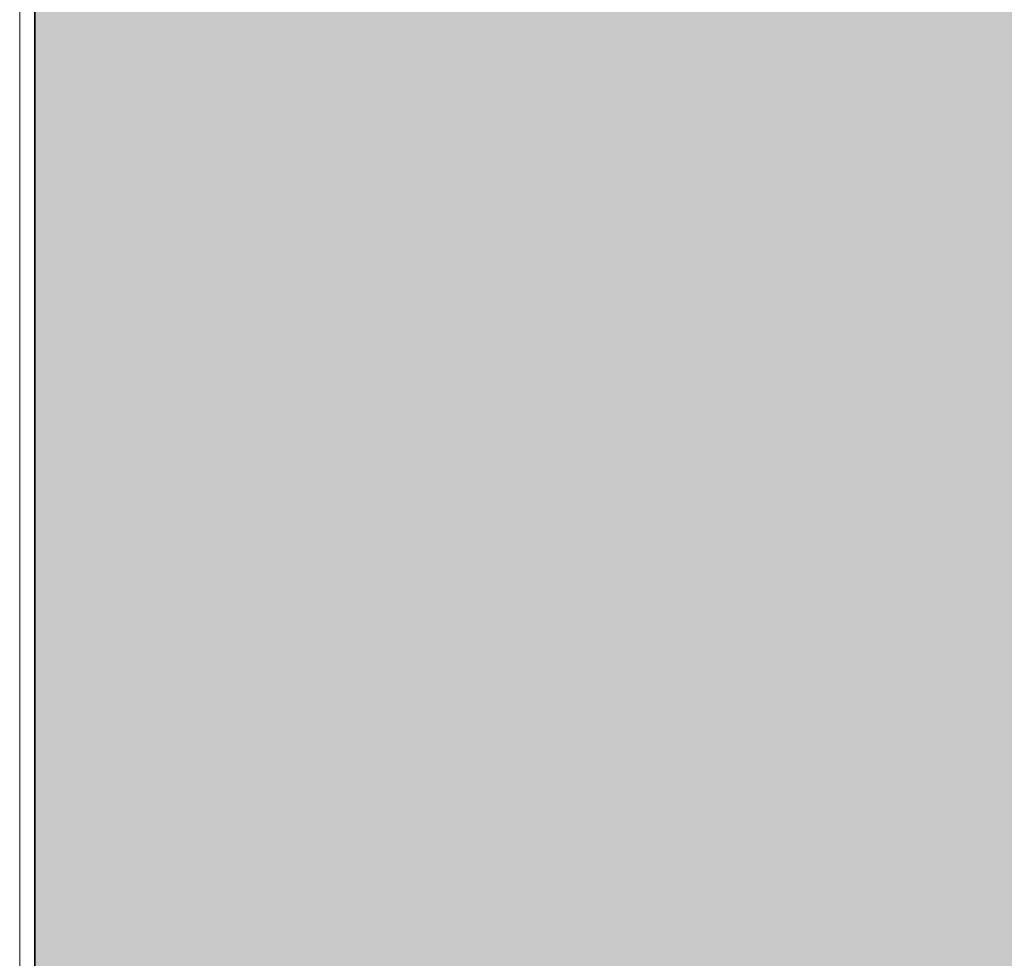
# Model space of a CAD drawing. Units: inches. Extents: x 2091 to 2899, y 967 to 2217.
# Tile 236 of 256: x 2203.116 to 2204.921, y 1153.969 to 1155.69. Entities that reach past the tile are written whole.
import ezdxf

# ---------------------------------------------------------------- set-up
doc = ezdxf.new("R2010")
doc.units = ezdxf.units.IN
doc.layers.add('A-GLAZ', color=4, linetype='Continuous', lineweight=18)
doc.layers.add('C-PROP', color=7, linetype='Continuous', lineweight=35)
doc.layers.add('A-WALL-PATT', color=141, linetype='Continuous', lineweight=13, true_color=0xadddf7)

# ---------------------------------------------------------------- blocks, each defined once
blk = doc.blocks.new('WIN-DOUBLE-LINE')
blk.add_line((0.0004, -0.0004), (0.0004, 80.8229))

msp = doc.modelspace()

# ---------------------------------------------------------------- hatches: boundary and pattern name
at = {"layer": 'A-WALL-PATT'}
h = msp.add_hatch(color=256, dxfattribs=at)
h.dxf.hatch_style = 1
h.paths.add_polyline_path([(2803.1436, 2050.9191), (2203.1436, 2050.9191), (2203.1436, 1090.9191), (2803.1436, 1090.9191)])
h.paths.add_polyline_path([(2635.7989, 1147.5405), (2674.5241, 1147.5405, 0.376086), (2678.5297, 1152.8802), (2678.5297, 1159.5565, 0.333335), (2674.5243, 1163.5618), (2674.5243, 1163.5619), (2674.5243, 1192.9344), (2635.806, 1192.9344), (2597.0876, 1192.9344), (2597.0876, 1163.5618, 0.333335), (2593.0823, 1159.5565), (2593.0823, 1152.8802, 0.376086), (2597.0879, 1147.5405)], flags=0)
h.paths.add_polyline_path([(2436.0104, 1278.2408, 0.000483), (2435.9526, 1278.215, -0.001328), (2435.9356, 1278.1117, -0.001711), (2436.1164, 1278.0408, 0.002185)], flags=0)
h.paths.add_polyline_path([(2794.1436, 1143.4191), (2794.1436, 1347.4191), (2543.3702, 1347.4191), (2543.3702, 1351.9191), (2794.1436, 1351.9191), (2794.1436, 1392.7136), (2793.9474, 1392.7136), (2793.9474, 1473.5369), (2794.1436, 1473.5369), (2794.1436, 1531.9191), (2650.1436, 1531.9191), (2650.1436, 1536.4191), (2794.1436, 1536.4191), (2794.1436, 1692.4191), (2609.3756, 1692.4191), (2609.3756, 1644.4191), (2604.8756, 1644.4191), (2604.8756, 1744.9191), (2609.3756, 1744.9191), (2609.3756, 1696.9191), (2794.1436, 1696.9191), (2794.1436, 1780.9191), (2609.6436, 1780.9191), (2493.8756, 1780.9191), (2493.8756, 1785.4191), (2609.6436, 1785.4191), (2794.1436, 1785.4191), (2794.1436, 1847.9388), (2793.9512, 1847.9388), (2793.9512, 1928.7622), (2794.1436, 1928.7622), (2794.1436, 1941.4191), (2614.1436, 1941.4191), (2614.1436, 1821.4191), (2609.6436, 1821.4191), (2609.6436, 1941.4191), (2392.1436, 1941.4191), (2392.1436, 1819.9191), (2387.6436, 1819.9191), (2387.6436, 1941.4191), (2212.1436, 1941.4191), (2212.1436, 1783.9191), (2392.1436, 1783.9191), (2392.1436, 1780.9191), (2212.1436, 1780.9191), (2212.1436, 1629.4191), (2387.6436, 1629.4191), (2387.6436, 1744.9191), (2392.1436, 1744.9191), (2392.1436, 1627.9191), (2317.1436, 1627.9191), (2317.1436, 1551.4191), (2317.1436, 1536.4191), (2459.3836, 1536.4191), (2459.3836, 1602.3965), (2463.8836, 1602.3965), (2463.8836, 1531.9191), (2456.6436, 1531.9191), (2456.6436, 1529.9191), (2452.1436, 1529.9191), (2452.1436, 1531.9191), (2312.6436, 1531.9191), (2312.6436, 1551.4191), (2306.1436, 1551.4191), (2306.1436, 1555.9191), (2308.1436, 1555.9191), (2308.1436, 1551.4191), (2312.6436, 1551.4191), (2312.6436, 1627.9191), (2212.1436, 1627.9191), (2212.1436, 1555.9191), (2270.1436, 1555.9191), (2270.1436, 1551.4191), (2212.1436, 1551.4191), (2212.1436, 1351.9191), (2272.1436, 1351.9191), (2272.1436, 1347.4191), (2212.1436, 1347.4191), (2212.1436, 1275.4191), (2308.1436, 1275.4191), (2308.1436, 1351.9191), (2452.1436, 1351.9191), (2452.1436, 1493.9191), (2456.6436, 1493.9191), (2456.6436, 1347.4191), (2312.6436, 1347.4191), (2312.6436, 1270.9191), (2212.1436, 1270.9191), (2212.1436, 1099.9191), (2281.2375, 1099.9191), (2282.871, 1110.9138), (2282.0083, 1116.9966), (2278.5577, 1121.4204), (2268.2056, 1128.0562), (2272.0876, 1128.0562), (2273.8129, 1131.927), (2279.4203, 1134.6919), (2285.0278, 1135.2449), (2287.6158, 1137.4568), (2288.0471, 1138.0098), (2289.3411, 1140.7747), (2291.0665, 1139.6687), (2292.3605, 1135.2449), (2295.3798, 1136.9038), (2296.2425, 1135.7979), (2297.1052, 1133.033), (2300.1246, 1138.0098), (2303.1439, 1138.0098), (2304.4379, 1135.7979), (2303.1439, 1133.586), (2306.5946, 1134.6919), (2307.8887, 1133.033), (2310.908, 1135.2449), (2313.9274, 1134.1389), (2315.6269, 1132.4271), (2308.32, 1117.5496), (2290.2038, 1109.8079), (2288.9098, 1103.1721), (2289.2723, 1099.9191), (2434.9182, 1099.9191), (2431.5932, 1124.7881), (2429.9302, 1169.5531), (2430.9272, 1240.5197), (2435.6589, 1238.1861), (2437.1352, 1196.5541), (2438.7982, 1143.9731), (2442.6782, 1111.9981), (2446.5582, 1099.9191), (2794.1436, 1099.9191), (2794.1436, 1138.9191), (2548.0324, 1138.9191), (2548.0324, 1143.4191), (2548.0324, 1148.8191), (2546.6685, 1148.0316), (2528.6857, 1179.1786, 0.256256), (2512.0324, 1148.8191), (2512.0324, 1143.4191), (2512.0324, 1138.9191), (2507.5324, 1138.9191), (2507.5324, 1143.4191), (2507.5324, 1148.8191, 0.256256), (2490.8792, 1179.1786), (2472.8964, 1148.0316), (2471.5324, 1148.8191), (2471.5324, 1143.4191), (2467.0324, 1143.4191), (2467.0324, 1269.9458, 0.039061), (2460.91, 1273.5801), (2467.0324, 1273.5801), (2467.0324, 1286.3254, 0.014511), (2465.2162, 1286.7619), (2467.0324, 1287.0526), (2467.0324, 1323.4191), (2471.5324, 1323.4191), (2471.5324, 1148.8191), (2489.5324, 1179.996), (2490.8964, 1179.2085), (2490.8792, 1179.1786, -0.256256), (2507.5324, 1148.8191), (2507.5324, 1143.4191), (2512.0324, 1143.4191), (2512.0324, 1148.8191, -0.256256), (2528.6857, 1179.1786), (2528.6685, 1179.2085), (2530.0324, 1179.996), (2548.0324, 1148.8191), (2548.0324, 1143.4191)], flags=16)
h.paths.add_polyline_path([(2607.7685, 1200.9451), (2607.7685, 1265.0306), (2597.0876, 1281.052), (2619.7846, 1281.052), (2627.7953, 1337.1269), (2635.7989, 1337.1269), (2643.8167, 1337.1269), (2651.8274, 1281.052), (2674.5243, 1281.052), (2663.8434, 1265.0306), (2663.8434, 1200.9451), (2635.806, 1200.9451)], flags=0)
edge = h.paths.add_edge_path(flags=0)
edge.add_ellipse((13303.8962, 1272.9987), major_axis=(-10595.313, 0), ratio=0.8423038701, start_angle=0.62823722, end_angle=0.6465541, ccw=False)
edge.add_ellipse((2711.7004, 1156.8527), major_axis=(2.2198, 0), ratio=0.842304, start_angle=111.5352, end_angle=180.6282, ccw=False)
edge.add_ellipse((13303.1563, 1272.9987), major_axis=(-10593.0263, 0), ratio=0.8423038695, start_angle=0.52827147, end_angle=0.6465541, ccw=False)
edge.add_line((2710.7646, 1175.3333), (2710.13, 1175.3333))
edge.add_ellipse((2710.13, 1176.5798), major_axis=(1.4798, 0), ratio=0.842304, start_angle=180, end_angle=270, ccw=False)
edge.add_line((2708.6501, 1176.5798), (2708.6501, 1200.7829))
edge.add_ellipse((2710.13, 1200.7829), major_axis=(1.4798, 0), ratio=0.842304, start_angle=90, end_angle=180, ccw=False)
edge.add_line((2710.13, 1202.0294), (2710.4651, 1202.0294))
edge.add_ellipse((13303.1563, 1272.9987), major_axis=(-10593.0263, 0), ratio=0.8423038695, start_angle=-0.09022909, end_angle=0.38386678, ccw=False)
edge.add_ellipse((2710.13, 1290.927), major_axis=(-1.4798, 0), ratio=0.842304, start_angle=0, end_angle=90, ccw=False)
edge.add_line((2708.6501, 1290.927), (2708.6501, 1315.1302))
edge.add_ellipse((2710.13, 1315.1302), major_axis=(-1.4798, 0), ratio=0.842304, start_angle=-90, end_angle=0, ccw=False)
edge.add_line((2710.13, 1316.3767), (2710.7063, 1316.3767))
edge.add_ellipse((3238.4017, 1296.2896), major_axis=(528.234, 0), ratio=0.84230387, start_angle=176.349572, end_angle=177.82005, ccw=False)
edge.add_ellipse((2775.063, 1071.4507), major_axis=(313.3078, 0), ratio=0.84230387, start_angle=102.125966, end_angle=103.780529, ccw=False)
edge.add_ellipse((2775.063, 1078.3057), major_axis=(-305.3029, 0), ratio=0.84230387, start_angle=-79.790461, end_angle=-77.555373, ccw=False)
edge.add_ellipse((2695.1418, 1541.9754), major_axis=(-250.9602, 0), ratio=0.84230387, start_angle=99.256566, end_angle=102.554933)
edge.add_line((2741.4103, 1334.2143), (2747.1325, 1337.3785))
edge.add_ellipse((2747.5386, 1336.8575), major_axis=(-0.7399, 0), ratio=0.842304, start_angle=270, end_angle=307.9331, ccw=False)
edge.add_ellipse((2747.5386, 1336.8575), major_axis=(-0.7399, 0), ratio=0.842304, start_angle=232.0669, end_angle=270, ccw=False)
edge.add_line((2747.9447, 1337.3785), (2753.6669, 1334.2143))
edge.add_ellipse((2799.9355, 1541.9754), major_axis=(250.9602, 0), ratio=0.84230387, start_angle=257.445067, end_angle=260.743434)
edge.add_ellipse((2720.0142, 1078.3057), major_axis=(305.3029, 0), ratio=0.84230387, start_angle=77.555373, end_angle=79.790461, ccw=False)
edge.add_ellipse((2720.0142, 1071.4507), major_axis=(-313.3078, 0), ratio=0.84230387, start_angle=256.219471, end_angle=257.874034, ccw=False)
edge.add_ellipse((2256.6755, 1296.2896), major_axis=(-528.234, 0), ratio=0.84230387, start_angle=182.17995, end_angle=183.650428, ccw=False)
edge.add_line((2784.3709, 1316.3767), (2784.9472, 1316.3767))
edge.add_ellipse((2784.9472, 1315.1302), major_axis=(1.4798, 0), ratio=0.842304, start_angle=0, end_angle=90, ccw=False)
edge.add_line((2786.4271, 1315.1302), (2786.4271, 1290.927))
edge.add_ellipse((2784.9472, 1290.927), major_axis=(1.4798, 0), ratio=0.842304, start_angle=270, end_angle=360, ccw=False)
edge.add_ellipse((-7808.0791, 1272.9987), major_axis=(10593.0263, 0), ratio=0.8423038695, start_angle=-0.38386678, end_angle=0.09022909, ccw=False)
edge.add_line((2784.6122, 1202.0294), (2784.9472, 1202.0294))
edge.add_ellipse((2784.9472, 1200.7829), major_axis=(1.4798, 0), ratio=0.842304, start_angle=0, end_angle=90, ccw=False)
edge.add_line((2786.4271, 1200.7829), (2786.4271, 1176.5798))
edge.add_ellipse((2784.9472, 1176.5798), major_axis=(-1.4798, 0), ratio=0.842304, start_angle=90, end_angle=180, ccw=False)
edge.add_line((2784.9472, 1175.3333), (2784.3126, 1175.3333))
edge.add_ellipse((-7808.0791, 1272.9987), major_axis=(10593.0263, 0), ratio=0.8423038695, start_angle=-0.6186432, end_angle=-0.52827147, ccw=False)
edge.add_ellipse((2783.3768, 1156.8527), major_axis=(-2.2198, 0), ratio=0.842304, start_angle=179.3718, end_angle=248.4648, ccw=False)
edge.add_ellipse((-7808.819, 1272.9987), major_axis=(-10595.313, 0), ratio=0.8423038658, start_angle=179.35344592, end_angle=179.3717628, ccw=False)
edge.add_ellipse((2780.2973, 1153.5008), major_axis=(-5.2464, 0), ratio=0.842304, start_angle=90, end_angle=179.3534, ccw=False)
edge.add_line((2780.2973, 1149.0817), (2714.7799, 1149.0817))
edge.add_ellipse((2714.7799, 1153.5008), major_axis=(5.2464, 0), ratio=0.842304, start_angle=180.6466, end_angle=270, ccw=False)
edge = h.paths.add_edge_path(flags=0)
edge.add_line((2718.1874, 1151.0078), (2718.1874, 1170.4724))
edge.add_ellipse((2721.1471, 1170.4724), major_axis=(-2.9597, 0), ratio=0.842304, start_angle=-90, end_angle=0, ccw=False)
edge.add_line((2721.1471, 1172.9653), (2773.9302, 1172.9653))
edge.add_ellipse((2773.9302, 1170.4724), major_axis=(-2.9597, 0), ratio=0.842304, start_angle=180, end_angle=270, ccw=False)
edge.add_line((2776.8899, 1170.4724), (2776.8899, 1151.0078))
edge.add_line((2776.8899, 1151.0078), (2718.1874, 1151.0078))
edge = h.paths.add_edge_path(flags=0)
edge.add_line((2718.1874, 1180.2342), (2718.1874, 1199.0578))
edge.add_ellipse((2747.5386, 1320.3986), major_axis=(147.0179, 0), ratio=0.84230387, start_angle=256.401865, end_angle=283.598135)
edge.add_line((2776.8899, 1199.0578), (2776.8899, 1180.2342))
edge.add_ellipse((2747.5386, 1301.575), major_axis=(147.0179, 0), ratio=0.84230387, start_angle=256.401865, end_angle=283.598135, ccw=False)
edge = h.paths.add_edge_path(flags=0)
edge.add_ellipse((13303.1563, 1272.9987), major_axis=(-10591.5465, 0), ratio=0.8423038696, start_angle=0.05559431, end_angle=0.37776419, ccw=False)
edge.add_line((2711.6169, 1262.7217), (2715.6674, 1249.4954))
edge.add_ellipse((6413.892, 1241.6919), major_axis=(-3698.2362, 0), ratio=0.84230387, start_angle=-0.1208974, end_angle=0.3640763)
edge.add_line((2715.761, 1218.1925), (2711.9343, 1203.1674))
edge = h.paths.add_edge_path(flags=0)
edge.add_line((2718.1874, 1251.0746), (2716.0025, 1267.4504))
edge.add_ellipse((2742.1512, 1202.1895), major_axis=(81.7726, 0), ratio=0.8423039, start_angle=94.277421, end_angle=111.834954, ccw=False)
edge.add_line((2737.0097, 1270.9306), (2758.0675, 1270.9306))
edge.add_ellipse((2752.9261, 1202.1895), major_axis=(81.7726, 0), ratio=0.8423039, start_angle=68.165046, end_angle=85.722579, ccw=False)
edge.add_line((2779.0747, 1267.4504), (2776.8899, 1251.0746))
edge.add_ellipse((2750.3381, 1187.8854), major_axis=(79.5797, 0), ratio=0.8423039, start_angle=67.208085, end_angle=85.12993)
edge.add_line((2756.0347, 1254.7437), (2739.0426, 1254.7437))
edge.add_ellipse((2744.7392, 1187.8854), major_axis=(79.5797, 0), ratio=0.8423039, start_angle=94.87007, end_angle=112.791915)
edge = h.paths.add_edge_path(flags=0)
edge.add_line((2783.1429, 1203.1674), (2779.3162, 1218.1925))
edge.add_ellipse((-918.8147, 1241.6919), major_axis=(3698.2362, 0), ratio=0.84230387, start_angle=-0.3640763, end_angle=0.1208974)
edge.add_line((2779.4098, 1249.4954), (2783.4604, 1262.7217))
edge.add_ellipse((-7808.0791, 1272.9987), major_axis=(-10591.5465, 0), ratio=0.8423038695, start_angle=179.62223581, end_angle=179.94440569, ccw=False)
edge = h.paths.add_edge_path(flags=0)
edge.add_ellipse((2734.2009, 1286.6904), major_axis=(-0.3566, 6.3401), ratio=0.603834, start_angle=89.00201, end_angle=253.65741, ccw=False)
edge.add_line((2730.369, 1286.5418), (2730.369, 1301.352))
edge.add_line((2730.369, 1301.352), (2735.9133, 1305.2148))
edge.add_ellipse((2736.3849, 1304.7346), major_axis=(0.7399, 0), ratio=0.842304, start_angle=90, end_angle=134.4802, ccw=False)
edge.add_line((2736.3849, 1305.3578), (2738.0328, 1305.3578))
edge.add_line((2738.0328, 1305.3578), (2738.0328, 1307.7079))
edge.add_ellipse((2794.2016, 1307.7079), major_axis=(56.1689, 0), ratio=0.8423039, start_angle=150.56143, end_angle=180, ccw=False)
edge.add_ellipse((2700.8756, 1307.7079), major_axis=(-56.1689, 0), ratio=0.8423039, start_angle=180, end_angle=209.43857, ccw=False)
edge.add_line((2757.0444, 1307.7079), (2757.0444, 1305.3578))
edge.add_line((2757.0444, 1305.3578), (2758.6923, 1305.3578))
edge.add_ellipse((2758.6923, 1304.7346), major_axis=(-0.7399, 0), ratio=0.842304, start_angle=225.5198, end_angle=270, ccw=False)
edge.add_line((2759.1639, 1305.2148), (2764.7082, 1301.352))
edge.add_line((2764.7082, 1301.352), (2764.7082, 1286.5418))
edge.add_ellipse((2760.8763, 1286.6904), major_axis=(0.3566, 6.3401), ratio=0.603834, start_angle=106.34259, end_angle=270.99799, ccw=False)
edge.add_line((2757.0444, 1285.7971), (2757.0444, 1307.7079))
edge.add_ellipse((2700.8756, 1307.7079), major_axis=(-56.1689, 0), ratio=0.8423039, start_angle=180, end_angle=209.43857)
edge.add_ellipse((2794.2016, 1307.7079), major_axis=(56.1689, 0), ratio=0.8423039, start_angle=150.56143, end_angle=180)
edge.add_line((2738.0328, 1307.7079), (2738.0328, 1285.7971))
h.paths.add_polyline_path([(2417.8123, 1104.4497), (2413.4923, 1102.5297), (2410.6123, 1103.9697), (2409.1723, 1106.3697), (2407.2523, 1107.3297), (2406.2923, 1109.7297), (2405.3323, 1114.0497), (2405.3323, 1117.8897), (2406.2923, 1120.1297), (2407.2523, 1119.8097), (2408.8483, 1118.3277), (2410.1739, 1119.4242), (2410.2113, 1120.4057), (2411.0407, 1121.4191), (2410.6993, 1119.8587), (2410.1739, 1119.4242), (2410.0885, 1117.1761), (2411.1328, 1116.2063), (2413.9723, 1119.3297), (2416.8523, 1120.7697), (2416.8697, 1120.7988), (2417.0351, 1119.4051), (2417.8962, 1118.1434), (2418.2923, 1118.3697), (2419.5444, 1120.0393), (2419.3609, 1118.3875), (2419.0321, 1119.3562), (2418.3989, 1118.5119), (2419.2523, 1114.5297), (2418.7941, 1107.1988)], flags=0)
h.paths.add_polyline_path([(2508.8702, 1347.4191), (2508.3702, 1347.4191), (2508.3702, 1351.9191), (2508.8702, 1351.9191)], flags=0)
h.paths.add_polyline_path([(2473.3702, 1347.4191), (2472.3702, 1347.4191), (2467.8702, 1347.4191), (2467.8702, 1455.4191), (2472.3702, 1455.4191), (2472.3702, 1352.4191), (2473.3702, 1352.4191)], flags=0)
h.paths.add_polyline_path([(2352.1062, 1217.4462), (2349.2262, 1218.8862), (2347.7862, 1221.2862), (2345.8662, 1222.2462), (2344.9062, 1224.6462), (2343.9462, 1228.9662), (2343.9462, 1232.8062), (2344.9062, 1235.0462), (2345.8662, 1234.7262), (2347.4623, 1233.2442), (2348.7879, 1234.3407), (2348.8252, 1235.3222), (2349.6547, 1236.3355), (2349.3132, 1234.7752), (2348.7879, 1234.3407), (2348.7024, 1232.0926), (2349.7468, 1231.1228), (2352.5862, 1234.2462), (2355.4662, 1235.6862), (2355.4837, 1235.7153), (2355.649, 1234.3216), (2356.5102, 1233.0599), (2356.9062, 1233.2862), (2358.1584, 1234.9558), (2357.9749, 1233.304), (2357.6461, 1234.2726), (2357.0129, 1233.4284), (2357.8662, 1229.4462), (2357.4081, 1222.1153), (2356.4262, 1219.3662)], flags=0)
h.paths.add_polyline_path([(2348.2968, 1112.2244), (2347.0138, 1112.3104), (2345.5298, 1114.1274), (2345.7318, 1115.8584), (2346.8118, 1116.9824), (2346.8118, 1114.6464), (2345.8668, 1114.2144), (2346.8798, 1114.3004)], flags=0)
h.paths.add_polyline_path([(2347.0138, 1110.9264), (2346.2718, 1110.4934), (2346.6098, 1111.1864)], flags=0)
h.paths.add_polyline_path([(2345.8668, 1118.1944), (2345.5298, 1117.3294), (2343.7078, 1118.0214), (2344.3828, 1118.6264)], flags=0)
h.paths.add_polyline_path([(2346.6768, 1109.2824), (2346.0698, 1108.0714), (2345.8668, 1110.0614)], flags=0)
h.paths.add_polyline_path([(2345.0568, 1119.7514), (2343.6398, 1119.7514), (2343.9778, 1121.1354)], flags=0)
h.paths.add_polyline_path([(2345.2598, 1116.5504), (2345.1248, 1115.8584), (2344.9218, 1115.6854), (2344.7198, 1116.3774)], flags=0)
h.paths.add_polyline_path([(2345.6648, 1112.3104), (2345.4618, 1111.5324), (2344.0448, 1111.9644), (2344.6518, 1112.5704)], flags=0)
h.paths.add_polyline_path([(2345.1918, 1113.3494), (2344.4498, 1113.8684), (2344.7198, 1114.3874)], flags=0)
h.paths.add_polyline_path([(2344.6518, 1116.8094), (2344.1798, 1115.6854), (2344.6518, 1115.3394), (2343.9098, 1114.9064), (2343.0328, 1115.9444), (2343.6398, 1116.4634)], flags=0)
h.paths.add_polyline_path([(2345.8668, 1106.6864), (2344.9898, 1105.5624), (2344.5168, 1106.6004)], flags=0)
h.paths.add_polyline_path([(2344.8548, 1110.0614), (2344.5168, 1109.2824), (2344.1128, 1109.7154)], flags=0)
h.paths.add_polyline_path([(2344.0448, 1113.5224), (2343.4378, 1113.0894), (2342.7628, 1113.9544)], flags=0)
h.paths.add_polyline_path([(2344.3148, 1111.0124), (2342.9648, 1110.3204), (2342.9648, 1111.0994)], flags=0)
h.paths.add_polyline_path([(2345.1248, 1104.6974), (2344.5848, 1103.7454), (2344.4498, 1104.2644)], flags=0)
h.paths.add_polyline_path([(2342.8298, 1121.2224), (2341.7498, 1120.5304), (2340.5358, 1121.0494), (2340.1308, 1121.8284), (2340.6708, 1122.9524), (2341.1428, 1121.8284), (2341.6148, 1122.0014)], flags=0)
h.paths.add_polyline_path([(2342.9648, 1119.7514), (2343.0328, 1118.4534), (2342.0878, 1118.0214), (2342.0198, 1119.4914)], flags=0)
h.paths.add_polyline_path([(2342.6948, 1116.8964), (2341.9528, 1116.6364), (2342.0198, 1117.3294)], flags=0)
h.paths.add_polyline_path([(2343.0328, 1112.2244), (2342.0198, 1111.7914), (2341.5478, 1112.2244), (2342.3578, 1113.3494)], flags=0)
h.paths.add_polyline_path([(2343.7748, 1104.4374), (2342.6278, 1102.8804), (2342.6948, 1104.6104), (2343.4378, 1105.1294)], flags=0)
h.paths.add_polyline_path([(2342.0198, 1115.0794), (2340.8058, 1115.5124), (2340.9408, 1116.3774)], flags=0)
h.paths.add_polyline_path([(2341.4808, 1120.0974), (2341.4808, 1119.4054), (2341.0758, 1119.5784), (2341.1428, 1120.0974)], flags=0)
h.paths.add_polyline_path([(2341.8178, 1114.4734), (2340.9408, 1113.0894), (2340.8058, 1114.5604)], flags=0)
h.paths.add_polyline_path([(2341.1428, 1118.5404), (2340.9408, 1116.9824), (2339.0508, 1117.6754), (2339.0508, 1118.6264)], flags=0)
h.paths.add_polyline_path([(2342.6948, 1101.6684), (2341.9528, 1101.8414), (2342.5598, 1102.3614)], flags=0)
h.paths.add_polyline_path([(2340.3328, 1119.6654), (2338.4438, 1119.5784), (2337.9038, 1120.3574), (2339.6578, 1120.6164)], flags=0)
h.paths.add_polyline_path([(2340.3328, 1115.3394), (2340.0628, 1113.6954), (2339.3878, 1115.3394)], flags=0)
h.paths.add_polyline_path([(2341.8178, 1103.8314), (2341.5478, 1102.8804), (2341.1428, 1103.6584)], flags=0)
h.paths.add_polyline_path([(2339.0508, 1122.8664), (2337.2958, 1121.8284), (2337.0938, 1123.1254), (2337.7688, 1123.8184)], flags=0)
h.paths.add_polyline_path([(2339.1178, 1121.7414), (2338.8478, 1121.2224), (2338.1738, 1121.0494), (2338.3758, 1121.5684)], flags=0)
h.paths.add_polyline_path([(2339.1858, 1119.3194), (2338.6458, 1118.7134), (2338.2408, 1118.1074), (2338.2408, 1118.8864)], flags=0)
h.paths.add_polyline_path([(2341.1428, 1101.9284), (2340.6028, 1101.2364), (2340.0628, 1101.8414), (2340.6028, 1102.3614)], flags=0)
h.paths.add_polyline_path([(2337.6338, 1117.7614), (2336.6208, 1118.2804), (2337.2958, 1118.9724)], flags=0)
h.paths.add_polyline_path([(2336.8238, 1119.5784), (2334.7988, 1118.9724), (2335.2038, 1120.3574), (2336.5538, 1120.8764)], flags=0)
h.paths.add_polyline_path([(2339.1178, 1100.4574), (2337.3638, 1100.5434), (2336.7558, 1101.2364)], flags=0)
h.paths.add_polyline_path([(2336.3508, 1122.4334), (2336.0138, 1121.9144), (2334.9338, 1122.4334), (2334.5288, 1123.4714), (2335.7438, 1122.7794)], flags=0)
h.paths.add_polyline_path([(2334.7318, 1120.8764), (2334.2588, 1120.3574), (2334.0568, 1120.7894), (2334.5968, 1121.3084)], flags=0)
h.paths.add_polyline_path([(2334.4618, 1122.1744), (2332.5718, 1121.3084), (2331.3568, 1122.1744), (2332.0998, 1122.8664)], flags=0)
h.paths.add_polyline_path([(2334.2588, 1118.5404), (2333.3818, 1118.4534), (2333.6518, 1119.3194)], flags=0)
h.paths.add_polyline_path([(2335.5418, 1102.2744), (2334.1918, 1102.6204), (2335.2718, 1103.3124)], flags=0)
h.paths.add_polyline_path([(2332.7068, 1119.6654), (2331.6948, 1120.4434), (2332.5048, 1120.7894)], flags=0)
h.paths.add_polyline_path([(2334.7318, 1101.1494), (2333.5168, 1101.5824), (2333.9888, 1101.7554)], flags=0)
h.paths.add_polyline_path([(2332.6398, 1116.6364), (2331.0868, 1116.2904), (2331.9648, 1118.1944)], flags=0)
h.paths.add_polyline_path([(2330.7498, 1121.5684), (2330.2768, 1120.2704), (2328.5228, 1119.3194), (2328.9948, 1121.0494)], flags=0)
h.paths.add_polyline_path([(2330.7498, 1118.6264), (2330.0078, 1117.5024), (2329.8728, 1118.0214)], flags=0)
h.paths.add_polyline_path([(2332.0998, 1102.3614), (2330.5468, 1102.0144), (2331.6948, 1102.9664)], flags=0)
h.paths.add_polyline_path([(2329.5348, 1113.6084), (2329.0628, 1112.3104), (2328.5898, 1113.3494)], flags=0)
h.paths.add_polyline_path([(2328.3878, 1117.8484), (2327.5098, 1116.5504), (2327.1728, 1117.7614)], flags=0)
h.paths.add_polyline_path([(2329.7378, 1106.5134), (2329.5348, 1105.3024), (2328.2528, 1106.0814)], flags=0)
h.paths.add_polyline_path([(2328.6578, 1114.3874), (2328.0498, 1114.1274), (2328.3198, 1114.9064)], flags=0)
h.paths.add_polyline_path([(2328.3198, 1112.2244), (2327.1058, 1112.1374), (2326.7008, 1112.6564)], flags=0)
h.paths.add_polyline_path([(2326.9028, 1115.2524), (2326.7008, 1114.1274), (2325.2158, 1113.6084), (2326.0928, 1115.3394)], flags=0)
h.paths.add_polyline_path([(2326.6328, 1108.3304), (2326.0928, 1107.3794), (2325.8908, 1108.5034), (2326.4978, 1109.1094)], flags=0)
h.paths.add_polyline_path([(2615.1436, 1531.9191), (2609.6436, 1531.9191), (2609.6436, 1620.4191), (2614.1436, 1620.4191), (2614.1436, 1536.4191), (2615.1436, 1536.4191)], flags=0)
h.paths.add_polyline_path([(2545.1436, 1563.4191), (2464.1436, 1563.4191), (2464.1436, 1632.4191), (2509.1436, 1632.4191), (2509.1436, 1627.9191), (2509.1436, 1603.9191), (2468.6436, 1603.9191), (2468.6436, 1567.9191), (2540.6436, 1567.9191), (2540.6436, 1591.9191), (2545.1436, 1591.9191)], flags=0)
h.paths.add_polyline_path([(2388.969, 1549.9857), (2357.4342, 1549.9857), (2357.4342, 1623.3608), (2399.3628, 1623.3608), (2435.6895, 1623.3608), (2435.5925, 1602.5593), (2435.5925, 1602.3965), (2388.969, 1602.3965)], flags=0)
h.paths.add_polyline_path([(2388.8806, 1555.8092), (2374.9044, 1555.8092), (2374.9044, 1600.5716), (2374.9044, 1615.4576), (2406.3509, 1615.4576), (2406.3509, 1618.9394), (2412.1743, 1615.4576), (2406.3509, 1611.9759), (2406.3509, 1615.4576), (2388.8806, 1615.4576)], flags=0)
h.paths.add_polyline_path([(2568.8756, 1644.4191), (2453.3756, 1644.4191), (2453.3756, 1785.4191), (2457.8756, 1785.4191), (2457.8756, 1648.9191), (2568.8756, 1648.9191)], flags=0)
h.paths.add_polyline_path([(2212.1436, 1945.9191), (2212.1436, 2041.9191), (2794.1436, 2041.9191), (2794.1436, 1945.9191)], flags=16)
h.paths.add_polyline_path([(2271.0827, 1964.3172), (2776.853, 1964.3172), (2776.853, 2037.1696), (2271.0827, 2037.1696)], flags=8)
h.paths.add_polyline_path([(2380.6493, 1536.8241), (2461.0408, 1536.8241), (2461.0408, 1554.6526), (2380.6493, 1554.6526)], flags=8)
h.paths.add_polyline_path([(2240.7557, 1609.7255), (2309.1858, 1609.7255), (2309.1858, 1617.6982), (2240.7557, 1617.6982)], flags=8)
h.paths.add_polyline_path([(2212.6773, 1313.5041), (2282.5915, 1313.5041), (2282.5915, 1322.7452), (2212.6773, 1322.7452)], flags=8)
h.paths.add_polyline_path([(2457.112, 1114.7786), (2558.4816, 1114.7786), (2558.4816, 1142.2197), (2457.112, 1142.2197)], flags=8)
h.paths.add_polyline_path([(2473.4423, 1273.0101), (2604.6412, 1273.0101), (2604.6412, 1318.3469), (2473.4423, 1318.3469)], flags=8)
h.paths.add_polyline_path([(2638.8763, 1626.9774), (2684.2504, 1627.9767), (2684.0385, 1637.5975), (2638.6644, 1636.5982)], flags=8)
h.paths.add_polyline_path([(2537.5906, 1453.7934), (2628.3895, 1453.7934), (2628.3895, 1475.3448), (2537.5906, 1475.3448)], flags=8)
h.paths.add_polyline_path([(2504.1376, 1714.6324), (2554.6472, 1714.6324), (2554.6472, 1730.2377), (2504.1376, 1730.2377)], flags=8)
h.paths.add_polyline_path([(2487.5012, 1575.6519), (2535.0971, 1575.6519), (2535.0971, 1598.3776), (2487.5012, 1598.3776)], flags=8)
h.paths.add_polyline_path([(2709.0994, 1735.7103), (2740.0166, 1735.7103), (2740.0166, 1749.9376), (2709.0994, 1749.9376)], flags=8)
h.paths.add_polyline_path([(2442.4384, 1792.1717), (2564.7288, 1792.1717), (2564.7288, 1842.0002), (2442.4384, 1842.0002)], flags=8)
h.paths.add_polyline_path([(2655.8158, 1809.6441), (2789.5201, 1806.6938), (2790.085, 1832.2916), (2656.3806, 1835.2419)], flags=8)
h.paths.add_polyline_path([(2234.8427, 1797.7201), (2368.5929, 1794.7689), (2369.1607, 1820.5041), (2235.4106, 1823.4554)], flags=8)
h.paths.add_polyline_path([(2245.1385, 1644.0063), (2398.4277, 1640.6239), (2398.9948, 1666.3248), (2245.7056, 1669.7073)], flags=8)
h.paths.add_polyline_path([(2306.1428, 1431.1685), (2413.7683, 1428.7937), (2414.3331, 1454.3915), (2306.7077, 1456.7664)], flags=8)
h.paths.add_polyline_path([(2306.8346, 1458.2331), (2393.3805, 1456.3234), (2393.9328, 1481.3544), (2307.3869, 1483.2641)], flags=8)

# ---------------------------------------------------------------- linework, layer by layer
at = {"layer": 'C-PROP'}
msp.add_lwpolyline([(2203.1436, 2050.9191), (2803.1436, 2050.9191), (2803.1436, 1090.9191), (2203.1436, 1090.9191)], close=True, dxfattribs=at)

# ---------------------------------------------------------------- block references
at = {"layer": 'A-GLAZ'}
msp.add_blockref('WIN-DOUBLE-LINE', (2203.1153, 1152.2475), dxfattribs=at)

doc.saveas('drawing.dxf')
